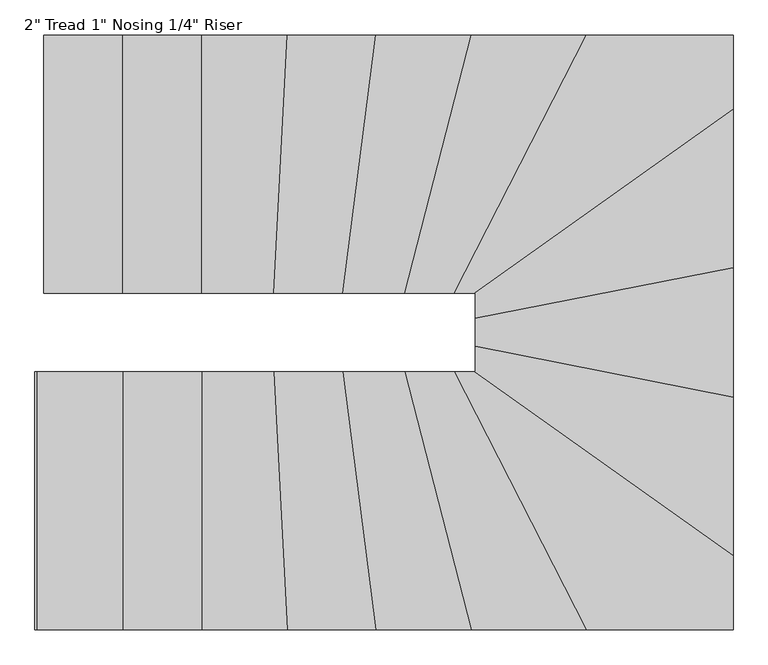
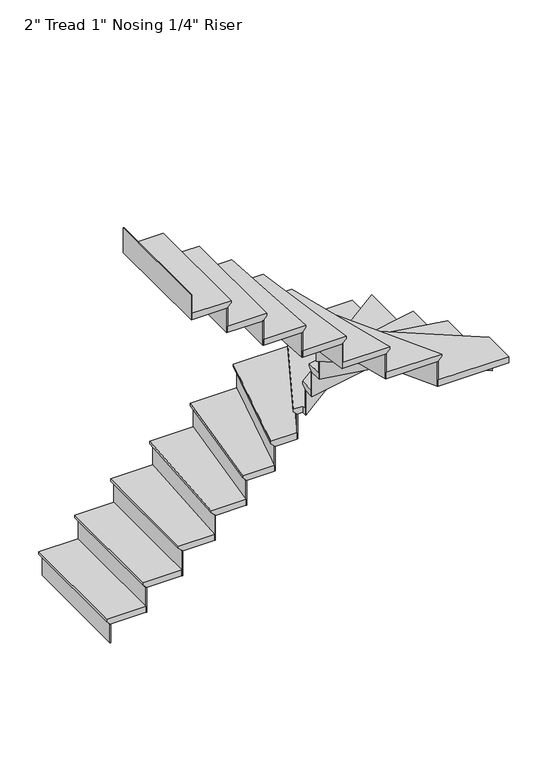
"""IFC4 building model written with IfcOpenShell, lengths in millimetres: stair flight geometry."""

from ifc_helpers import new_model, si_unit, origin, place, context, project, spatial, faceted_brep, source, transform, mapped, element, save


def stair_flight_27d53fa0(model_context):
    return source(origin(), model_context, "Body", "Brep", [
        faceted_brep([(306.9570026, -4376.7064015, 6584.95), (306.9570026, -4376.7064015, 6604.0), (306.9570026, -3462.3064015, 6604.0), (306.9570026, -3462.3064015, 6584.95), (332.3570026, -4376.7064015, 6559.55), (332.3570026, -3462.3064015, 6559.55), (611.7570026, -4376.7064015, 6604.0), (611.7570026, -3462.3064015, 6604.0), (332.3570026, -3462.3064015, 6553.2), (611.7570026, -3462.3064015, 6553.2), (611.7570026, -4376.7064015, 6553.2), (332.3570026, -4376.7064015, 6553.2)], [[[0, 1, 2, 3]], [[4, 0, 3, 5]], [[2, 1, 6, 7]], [[8, 9, 10, 11]], [[2, 7, 9, 8, 5, 3]], [[8, 11, 4, 5]], [[6, 1, 0, 4, 11, 10]], [[7, 6, 10, 9]]]),
        faceted_brep([(332.3570026, -4376.7064015, 6553.2), (332.3570026, -4376.7064015, 6400.8), (338.7070026, -4376.7064015, 6400.8), (338.7070026, -4376.7064015, 6553.2), (332.3570026, -3462.3064015, 6553.2), (338.7070026, -3462.3064015, 6553.2), (338.7070026, -3462.3064015, 6400.8), (332.3570026, -3462.3064015, 6400.8)], [[[0, 1, 2, 3]], [[4, 5, 6, 7]], [[1, 0, 4, 7]], [[2, 1, 7, 6]], [[3, 2, 6, 5]], [[0, 3, 5, 4]]]),
        faceted_brep([(611.7570026, -4376.7064015, 6756.4), (611.7570026, -4376.7064015, 6553.2), (618.1070026, -4376.7064015, 6553.2), (618.1070026, -4376.7064015, 6756.4), (611.7570026, -3462.3064015, 6756.4), (618.1070026, -3462.3064015, 6756.4), (618.1070026, -3462.3064015, 6553.2), (611.7570026, -3462.3064015, 6553.2)], [[[0, 1, 2, 3]], [[4, 5, 6, 7]], [[1, 0, 4, 7]], [[2, 1, 7, 6]], [[3, 2, 6, 5]], [[0, 3, 5, 4]]]),
        faceted_brep([(586.3570026, -3462.3064015, 6807.2), (586.3570026, -4376.7064015, 6807.2), (891.1570026, -4376.7064015, 6807.2), (891.1570026, -3462.3064015, 6807.2), (611.7570026, -3462.3064015, 6756.4), (891.1570026, -3462.3064015, 6756.4), (891.1570026, -4376.7064015, 6756.4), (611.7570026, -4376.7064015, 6756.4), (611.7570026, -3462.3064015, 6762.75), (586.3570026, -3462.3064015, 6788.15), (611.7570026, -4376.7064015, 6762.75), (586.3570026, -4376.7064015, 6788.15)], [[[0, 1, 2, 3]], [[4, 5, 6, 7]], [[0, 3, 5, 4, 8, 9]], [[4, 7, 10, 8]], [[2, 1, 11, 10, 7, 6]], [[3, 2, 6, 5]], [[11, 1, 0, 9]], [[10, 11, 9, 8]]]),
        faceted_brep([(891.1570026, -4376.7064015, 6959.6), (891.1570026, -4376.7064015, 6756.4), (897.5070026, -4376.7064015, 6756.4), (897.5070026, -4376.7064015, 6959.6), (891.1570026, -3462.3064015, 6959.6), (897.5070026, -3462.3064015, 6959.6), (897.5070026, -3462.3064015, 6756.4), (891.1570026, -3462.3064015, 6756.4)], [[[0, 1, 2, 3]], [[4, 5, 6, 7]], [[1, 0, 4, 7]], [[2, 1, 7, 6]], [[3, 2, 6, 5]], [[0, 3, 5, 4]]]),
        faceted_brep([(865.7570026, -3462.3064015, 7010.4), (865.7570026, -4376.7064015, 7010.4), (1146.824164, -4376.7064015, 7010.4), (1194.3584344, -3462.3064015, 7010.4), (891.1570026, -3462.3064015, 6959.6), (1194.3584344, -3462.3064015, 6959.6), (1146.824164, -4376.7064015, 6959.6), (891.1570026, -4376.7064015, 6959.6), (891.1570026, -3462.3064015, 6965.95), (865.7570026, -3462.3064015, 6991.35), (891.1570026, -4376.7064015, 6965.95), (865.7570026, -4376.7064015, 6991.35)], [[[0, 1, 2, 3]], [[4, 5, 6, 7]], [[0, 3, 5, 4, 8, 9]], [[4, 7, 10, 8]], [[2, 1, 11, 10, 7, 6]], [[3, 2, 6, 5]], [[11, 1, 0, 9]], [[10, 11, 9, 8]]]),
        faceted_brep([(1146.824164, -4376.7064015, 7162.8), (1146.824164, -4376.7064015, 6959.6), (1153.1827382, -4376.7064015, 6959.6), (1153.1827382, -4376.7064015, 7162.8), (1194.3584344, -3462.3064015, 7162.8), (1200.7170086, -3462.3064015, 7162.8), (1200.7170086, -3462.3064015, 6959.6), (1194.3584344, -3462.3064015, 6959.6)], [[[0, 1, 2, 3]], [[4, 5, 6, 7]], [[1, 0, 4, 7]], [[2, 1, 7, 6]], [[3, 2, 6, 5]], [[0, 3, 5, 4]]]),
        faceted_brep([(1168.9241378, -3462.3064015, 7213.6), (1121.3898673, -4376.7064015, 7213.6), (1390.9908638, -4376.7064015, 7213.6), (1509.3469155, -3462.3064015, 7213.6), (1194.3584344, -3462.3064015, 7162.8), (1509.3469155, -3462.3064015, 7162.8), (1390.9908638, -4376.7064015, 7162.8), (1146.824164, -4376.7064015, 7162.8), (1194.3584344, -3462.3064015, 7169.15), (1168.9241378, -3462.3064015, 7194.55), (1146.824164, -4376.7064015, 7169.15), (1121.3898673, -4376.7064015, 7194.55)], [[[0, 1, 2, 3]], [[4, 5, 6, 7]], [[0, 3, 5, 4, 8, 9]], [[4, 7, 10, 8]], [[2, 1, 11, 10, 7, 6]], [[3, 2, 6, 5]], [[11, 1, 0, 9]], [[10, 11, 9, 8]]]),
        faceted_brep([(1390.9908638, -4376.7064015, 7366.0), (1390.9908638, -4376.7064015, 7162.8), (1397.3938356, -4376.7064015, 7162.8), (1397.3938356, -4376.7064015, 7366.0), (1509.3469155, -3462.3064015, 7366.0), (1515.7498873, -3462.3064015, 7366.0), (1515.7498873, -3462.3064015, 7162.8), (1509.3469155, -3462.3064015, 7162.8)], [[[0, 1, 2, 3]], [[4, 5, 6, 7]], [[1, 0, 4, 7]], [[2, 1, 7, 6]], [[3, 2, 6, 5]], [[0, 3, 5, 4]]]),
        faceted_brep([(1483.7350284, -3462.3064015, 7416.8), (1365.3789767, -4376.7064015, 7416.8), (1612.6180863, -4376.7064015, 7416.8), (1847.7485337, -3462.3064015, 7416.8), (1509.3469155, -3462.3064015, 7366.0), (1847.7485337, -3462.3064015, 7366.0), (1612.6180863, -4376.7064015, 7366.0), (1390.9908638, -4376.7064015, 7366.0), (1509.3469155, -3462.3064015, 7372.35), (1483.7350284, -3462.3064015, 7397.75), (1390.9908638, -4376.7064015, 7372.35), (1365.3789767, -4376.7064015, 7397.75)], [[[0, 1, 2, 3]], [[4, 5, 6, 7]], [[0, 3, 5, 4, 8, 9]], [[4, 7, 10, 8]], [[2, 1, 11, 10, 7, 6]], [[3, 2, 6, 5]], [[11, 1, 0, 9]], [[10, 11, 9, 8]]]),
        faceted_brep([(1612.6180863, -4376.7064015, 7569.2), (1612.6180863, -4376.7064015, 7366.0), (1619.1746632, -4376.7064015, 7366.0), (1619.1746632, -4376.7064015, 7569.2), (1847.7485337, -3462.3064015, 7569.2), (1854.3051106, -3462.3064015, 7569.2), (1854.3051106, -3462.3064015, 7366.0), (1847.7485337, -3462.3064015, 7366.0)], [[[0, 1, 2, 3]], [[4, 5, 6, 7]], [[1, 0, 4, 7]], [[2, 1, 7, 6]], [[3, 2, 6, 5]], [[0, 3, 5, 4]]]),
        faceted_brep([(1821.5222263, -3462.3064015, 7620.0), (1586.3917788, -4376.7064015, 7620.0), (1788.9647224, -4376.7064015, 7620.0), (2257.7893437, -3462.3064015, 7620.0), (1847.7485337, -3462.3064015, 7569.2), (2257.7893437, -3462.3064015, 7569.2), (1788.9647224, -4376.7064015, 7569.2), (1612.6180863, -4376.7064015, 7569.2), (1847.7485337, -3462.3064015, 7575.55), (1821.5222263, -3462.3064015, 7600.95), (1612.6180863, -4376.7064015, 7575.55), (1586.3917788, -4376.7064015, 7600.95)], [[[0, 1, 2, 3]], [[4, 5, 6, 7]], [[0, 3, 5, 4, 8, 9]], [[4, 7, 10, 8]], [[2, 1, 11, 10, 7, 6]], [[3, 2, 6, 5]], [[11, 1, 0, 9]], [[10, 11, 9, 8]]]),
        faceted_brep([(1788.9647224, -4376.7064015, 7772.4), (1788.9647224, -4376.7064015, 7569.2), (1796.1007055, -4376.7064015, 7569.2), (1796.1007055, -4376.7064015, 7772.4), (2257.7893437, -3462.3064015, 7772.4), (2264.9253269, -3462.3064015, 7772.4), (2264.9253269, -3462.3064015, 7569.2), (2257.7893437, -3462.3064015, 7569.2)], [[[0, 1, 2, 3]], [[4, 5, 6, 7]], [[1, 0, 4, 7]], [[2, 1, 7, 6]], [[3, 2, 6, 5]], [[0, 3, 5, 4]]]),
        faceted_brep([(2749.0886944, -3755.9875352, 7823.2), (2749.0886944, -3462.3064015, 7823.2), (2229.2454112, -3462.3064015, 7823.2), (1760.4207899, -4376.7064015, 7823.2), (1834.6886944, -4376.7064015, 7823.2), (1834.6886944, -4406.2614844, 7823.2), (2749.0886944, -3462.3064015, 7772.4), (2749.0886944, -3755.9875352, 7772.4), (1834.6886944, -4406.2614844, 7772.4), (1834.6886944, -4376.7064015, 7772.4), (1788.9647224, -4376.7064015, 7772.4), (2257.7893437, -3462.3064015, 7772.4), (2257.7893437, -3462.3064015, 7778.75), (2229.2454112, -3462.3064015, 7804.15), (1788.9647224, -4376.7064015, 7778.75), (1760.4207899, -4376.7064015, 7804.15)], [[[0, 1, 2, 3, 4, 5]], [[6, 7, 8, 9, 10, 11]], [[1, 0, 7, 6]], [[2, 1, 6, 11, 12, 13]], [[11, 10, 14, 12]], [[4, 3, 15, 14, 10, 9]], [[5, 4, 9, 8]], [[0, 5, 8, 7]], [[15, 3, 2, 13]], [[14, 15, 13, 12]]]),
        faceted_brep([(1834.6886944, -4406.2614844, 7975.6), (1834.6886944, -4406.2614844, 7772.4), (1834.6886944, -4414.0534592, 7772.4), (1834.6886944, -4414.0534592, 7975.6), (2749.0886944, -3755.9875352, 7975.6), (2749.0886944, -3763.77951, 7975.6), (2749.0886944, -3763.77951, 7772.4), (2749.0886944, -3755.9875352, 7772.4)], [[[0, 1, 2, 3]], [[4, 5, 6, 7]], [[1, 0, 4, 7]], [[2, 1, 7, 6]], [[3, 2, 6, 5]], [[0, 3, 5, 4]]]),
        faceted_brep([(2749.0886944, -3724.819636, 8026.4), (1834.6886944, -4375.0935852, 8026.4), (1834.6886944, -4492.7155714, 8026.4), (2749.0886944, -4312.4747151, 8026.4), (2749.0886944, -3755.9875352, 7975.6), (2749.0886944, -4312.4747151, 7975.6), (1834.6886944, -4492.7155714, 7975.6), (1834.6886944, -4406.2614844, 7975.6), (2749.0886944, -3755.9875352, 7981.95), (2749.0886944, -3724.819636, 8007.35), (1834.6886944, -4406.2614844, 7981.95), (1834.6886944, -4375.0935852, 8007.35)], [[[0, 1, 2, 3]], [[4, 5, 6, 7]], [[0, 3, 5, 4, 8, 9]], [[4, 7, 10, 8]], [[2, 1, 11, 10, 7, 6]], [[3, 2, 6, 5]], [[11, 1, 0, 9]], [[10, 11, 9, 8]]]),
        faceted_brep([(1834.6886944, -4492.7155714, 8178.8), (1834.6886944, -4492.7155714, 7975.6), (1834.6886944, -4499.1877569, 7975.6), (1834.6886944, -4499.1877569, 8178.8), (2749.0886944, -4312.4747151, 8178.8), (2749.0886944, -4318.9469005, 8178.8), (2749.0886944, -4318.9469005, 7975.6), (2749.0886944, -4312.4747151, 7975.6)], [[[0, 1, 2, 3]], [[4, 5, 6, 7]], [[1, 0, 4, 7]], [[2, 1, 7, 6]], [[3, 2, 6, 5]], [[0, 3, 5, 4]]]),
        faceted_brep([(2749.0886944, -4286.5859733, 8229.6), (1834.6886944, -4466.8268297, 8229.6), (1834.6886944, -4591.8747151, 8229.6), (2749.0886944, -4772.1155714, 8229.6), (2749.0886944, -4312.4747151, 8178.8), (2749.0886944, -4772.1155714, 8178.8), (1834.6886944, -4591.8747151, 8178.8), (1834.6886944, -4492.7155714, 8178.8), (2749.0886944, -4312.4747151, 8185.15), (2749.0886944, -4286.5859733, 8210.55), (1834.6886944, -4492.7155714, 8185.15), (1834.6886944, -4466.8268297, 8210.55)], [[[0, 1, 2, 3]], [[4, 5, 6, 7]], [[0, 3, 5, 4, 8, 9]], [[4, 7, 10, 8]], [[2, 1, 11, 10, 7, 6]], [[3, 2, 6, 5]], [[11, 1, 0, 9]], [[10, 11, 9, 8]]]),
        faceted_brep([(1834.6886944, -4591.8747151, 8382.0), (1834.6886944, -4591.8747151, 8178.8), (1834.6886944, -4598.3469005, 8178.8), (1834.6886944, -4598.3469005, 8382.0), (2749.0886944, -4772.1155714, 8382.0), (2749.0886944, -4778.5877569, 8382.0), (2749.0886944, -4778.5877569, 8178.8), (2749.0886944, -4772.1155714, 8178.8)], [[[0, 1, 2, 3]], [[4, 5, 6, 7]], [[1, 0, 4, 7]], [[2, 1, 7, 6]], [[3, 2, 6, 5]], [[0, 3, 5, 4]]]),
        faceted_brep([(2749.0886944, -4746.2268297, 8432.8), (1834.6886944, -4565.9859733, 8432.8), (1834.6886944, -4656.1064015, 8432.8), (1788.5932199, -4656.1064015, 8432.8), (2749.0886944, -5339.1610662, 8432.8), (2749.0886944, -4772.1155714, 8382.0), (2749.0886944, -5339.1610662, 8382.0), (1788.5932199, -4656.1064015, 8382.0), (1834.6886944, -4656.1064015, 8382.0), (1834.6886944, -4591.8747151, 8382.0), (2749.0886944, -4772.1155714, 8388.35), (2749.0886944, -4746.2268297, 8413.75), (1834.6886944, -4591.8747151, 8388.35), (1834.6886944, -4565.9859733, 8413.75)], [[[0, 1, 2, 3, 4]], [[5, 6, 7, 8, 9]], [[0, 4, 6, 5, 10, 11]], [[5, 9, 12, 10]], [[2, 1, 13, 12, 9, 8]], [[3, 2, 8, 7]], [[4, 3, 7, 6]], [[13, 1, 0, 11]], [[12, 13, 11, 10]]]),
        faceted_brep([(1788.5932199, -4656.1064015, 8585.2), (1788.5932199, -4656.1064015, 8382.0), (1777.6363274, -4656.1064015, 8382.0), (1777.6363274, -4656.1064015, 8585.2), (2749.0886944, -5339.1610662, 8585.2), (2749.0886944, -5346.953041, 8585.2), (2749.0886944, -5346.953041, 8382.0), (2749.0886944, -5339.1610662, 8382.0)], [[[0, 1, 2, 3]], [[4, 5, 6, 7]], [[1, 0, 4, 7]], [[2, 1, 7, 6]], [[3, 2, 6, 5]], [[0, 3, 5, 4]]]),
        faceted_brep([(2200.7014787, -5570.5064015, 8636.0), (2749.0886944, -5570.5064015, 8636.0), (2749.0886944, -5307.993167, 8636.0), (1832.4207899, -4656.1064015, 8636.0), (1731.8768573, -4656.1064015, 8636.0), (2749.0886944, -5570.5064015, 8585.2), (2200.7014787, -5570.5064015, 8585.2), (1731.8768573, -4656.1064015, 8585.2), (1788.5932199, -4656.1064015, 8585.2), (2749.0886944, -5339.1610662, 8585.2), (2749.0886944, -5339.1610662, 8591.55), (2749.0886944, -5307.993167, 8616.95), (1788.5932199, -4656.1064015, 8591.55), (1832.4207899, -4656.1064015, 8616.95)], [[[0, 1, 2, 3, 4]], [[5, 6, 7, 8, 9]], [[1, 0, 6, 5]], [[2, 1, 5, 9, 10, 11]], [[9, 8, 12, 10]], [[4, 3, 13, 12, 8, 7]], [[0, 4, 7, 6]], [[13, 3, 2, 11]], [[12, 13, 11, 10]]]),
        faceted_brep([(1731.8768573, -4656.1064015, 8788.4), (1731.8768573, -4656.1064015, 8585.2), (1724.7408742, -4656.1064015, 8585.2), (1724.7408742, -4656.1064015, 8788.4), (2200.7014787, -5570.5064015, 8788.4), (2193.5654955, -5570.5064015, 8788.4), (2193.5654955, -5570.5064015, 8585.2), (2200.7014787, -5570.5064015, 8585.2)], [[[0, 1, 2, 3]], [[4, 5, 6, 7]], [[1, 0, 4, 7]], [[2, 1, 7, 6]], [[3, 2, 6, 5]], [[0, 3, 5, 4]]]),
        faceted_brep([(2229.2454112, -5570.5064015, 8839.2), (1760.4207899, -4656.1064015, 8839.2), (1560.1654714, -4656.1064015, 8839.2), (1795.2959188, -5570.5064015, 8839.2), (2200.7014787, -5570.5064015, 8788.4), (1795.2959188, -5570.5064015, 8788.4), (1560.1654714, -4656.1064015, 8788.4), (1731.8768573, -4656.1064015, 8788.4), (2200.7014787, -5570.5064015, 8794.75), (2229.2454112, -5570.5064015, 8820.15), (1731.8768573, -4656.1064015, 8794.75), (1760.4207899, -4656.1064015, 8820.15)], [[[0, 1, 2, 3]], [[4, 5, 6, 7]], [[0, 3, 5, 4, 8, 9]], [[4, 7, 10, 8]], [[2, 1, 11, 10, 7, 6]], [[3, 2, 6, 5]], [[11, 1, 0, 9]], [[10, 11, 9, 8]]]),
        faceted_brep([(1560.1654714, -4656.1064015, 8991.6), (1560.1654714, -4656.1064015, 8788.4), (1553.6088945, -4656.1064015, 8788.4), (1553.6088945, -4656.1064015, 8991.6), (1795.2959188, -5570.5064015, 8991.6), (1788.7393419, -5570.5064015, 8991.6), (1788.7393419, -5570.5064015, 8788.4), (1795.2959188, -5570.5064015, 8788.4)], [[[0, 1, 2, 3]], [[4, 5, 6, 7]], [[1, 0, 4, 7]], [[2, 1, 7, 6]], [[3, 2, 6, 5]], [[0, 3, 5, 4]]]),
        faceted_brep([(1821.5222263, -5570.5064015, 9042.4), (1586.3917788, -4656.1064015, 9042.4), (1339.7670896, -4656.1064015, 9042.4), (1458.1231413, -5570.5064015, 9042.4), (1795.2959188, -5570.5064015, 8991.6), (1458.1231413, -5570.5064015, 8991.6), (1339.7670896, -4656.1064015, 8991.6), (1560.1654714, -4656.1064015, 8991.6), (1795.2959188, -5570.5064015, 8997.95), (1821.5222263, -5570.5064015, 9023.35), (1560.1654714, -4656.1064015, 8997.95), (1586.3917788, -4656.1064015, 9023.35)], [[[0, 1, 2, 3]], [[4, 5, 6, 7]], [[0, 3, 5, 4, 8, 9]], [[4, 7, 10, 8]], [[2, 1, 11, 10, 7, 6]], [[3, 2, 6, 5]], [[11, 1, 0, 9]], [[10, 11, 9, 8]]]),
        faceted_brep([(1339.7670896, -4656.1064015, 9194.8), (1339.7670896, -4656.1064015, 8991.6), (1333.3641178, -4656.1064015, 8991.6), (1333.3641178, -4656.1064015, 9194.8), (1458.1231413, -5570.5064015, 9194.8), (1451.7201695, -5570.5064015, 9194.8), (1451.7201695, -5570.5064015, 8991.6), (1458.1231413, -5570.5064015, 8991.6)], [[[0, 1, 2, 3]], [[4, 5, 6, 7]], [[1, 0, 4, 7]], [[2, 1, 7, 6]], [[3, 2, 6, 5]], [[0, 3, 5, 4]]]),
        faceted_brep([(1483.7350284, -5570.5064015, 9245.6), (1365.3789767, -4656.1064015, 9245.6), (1095.9555707, -4656.1064015, 9245.6), (1143.4898411, -5570.5064015, 9245.6), (1458.1231413, -5570.5064015, 9194.8), (1143.4898411, -5570.5064015, 9194.8), (1095.9555707, -4656.1064015, 9194.8), (1339.7670896, -4656.1064015, 9194.8), (1458.1231413, -5570.5064015, 9201.15), (1483.7350284, -5570.5064015, 9226.55), (1339.7670896, -4656.1064015, 9201.15), (1365.3789767, -4656.1064015, 9226.55)], [[[0, 1, 2, 3]], [[4, 5, 6, 7]], [[0, 3, 5, 4, 8, 9]], [[4, 7, 10, 8]], [[2, 1, 11, 10, 7, 6]], [[3, 2, 6, 5]], [[11, 1, 0, 9]], [[10, 11, 9, 8]]]),
        faceted_brep([(1095.9555707, -4656.1064015, 9398.0), (1095.9555707, -4656.1064015, 9194.8), (1089.5969965, -4656.1064015, 9194.8), (1089.5969965, -4656.1064015, 9398.0), (1143.4898411, -5570.5064015, 9398.0), (1137.1312669, -5570.5064015, 9398.0), (1137.1312669, -5570.5064015, 9194.8), (1143.4898411, -5570.5064015, 9194.8)], [[[0, 1, 2, 3]], [[4, 5, 6, 7]], [[1, 0, 4, 7]], [[2, 1, 7, 6]], [[3, 2, 6, 5]], [[0, 3, 5, 4]]]),
        faceted_brep([(1168.9241378, -5570.5064015, 9448.8), (1121.3898673, -4656.1064015, 9448.8), (840.3570026, -4656.1064015, 9448.8), (840.3570026, -5570.5064015, 9448.8), (1143.4898411, -5570.5064015, 9398.0), (840.3570026, -5570.5064015, 9398.0), (840.3570026, -4656.1064015, 9398.0), (1095.9555707, -4656.1064015, 9398.0), (1143.4898411, -5570.5064015, 9404.35), (1168.9241378, -5570.5064015, 9429.75), (1095.9555707, -4656.1064015, 9404.35), (1121.3898673, -4656.1064015, 9429.75)], [[[0, 1, 2, 3]], [[4, 5, 6, 7]], [[0, 3, 5, 4, 8, 9]], [[4, 7, 10, 8]], [[2, 1, 11, 10, 7, 6]], [[3, 2, 6, 5]], [[11, 1, 0, 9]], [[10, 11, 9, 8]]]),
        faceted_brep([(840.3570026, -4656.1064015, 9601.2), (840.3570026, -4656.1064015, 9398.0), (834.0070026, -4656.1064015, 9398.0), (834.0070026, -4656.1064015, 9601.2), (840.3570026, -5570.5064015, 9601.2), (834.0070026, -5570.5064015, 9601.2), (834.0070026, -5570.5064015, 9398.0), (840.3570026, -5570.5064015, 9398.0)], [[[0, 1, 2, 3]], [[4, 5, 6, 7]], [[1, 0, 4, 7]], [[2, 1, 7, 6]], [[3, 2, 6, 5]], [[0, 3, 5, 4]]]),
        faceted_brep([(865.7570026, -5570.5064015, 9652.0), (865.7570026, -4656.1064015, 9652.0), (560.9570026, -4656.1064015, 9652.0), (560.9570026, -5570.5064015, 9652.0), (840.3570026, -5570.5064015, 9601.2), (560.9570026, -5570.5064015, 9601.2), (560.9570026, -4656.1064015, 9601.2), (840.3570026, -4656.1064015, 9601.2), (840.3570026, -5570.5064015, 9607.55), (865.7570026, -5570.5064015, 9632.95), (840.3570026, -4656.1064015, 9607.55), (865.7570026, -4656.1064015, 9632.95)], [[[0, 1, 2, 3]], [[4, 5, 6, 7]], [[0, 3, 5, 4, 8, 9]], [[4, 7, 10, 8]], [[2, 1, 11, 10, 7, 6]], [[3, 2, 6, 5]], [[11, 1, 0, 9]], [[10, 11, 9, 8]]]),
        faceted_brep([(560.9570026, -4656.1064015, 9804.4), (560.9570026, -4656.1064015, 9601.2), (554.6070026, -4656.1064015, 9601.2), (554.6070026, -4656.1064015, 9804.4), (560.9570026, -5570.5064015, 9804.4), (554.6070026, -5570.5064015, 9804.4), (554.6070026, -5570.5064015, 9601.2), (560.9570026, -5570.5064015, 9601.2)], [[[0, 1, 2, 3]], [[4, 5, 6, 7]], [[1, 0, 4, 7]], [[2, 1, 7, 6]], [[3, 2, 6, 5]], [[0, 3, 5, 4]]]),
        faceted_brep([(281.5570026, -4656.1064015, 10007.6), (281.5570026, -4656.1064015, 9804.4), (275.2070026, -4656.1064015, 9804.4), (275.2070026, -4656.1064015, 10007.6), (281.5570026, -5570.5064015, 10007.6), (275.2070026, -5570.5064015, 10007.6), (275.2070026, -5570.5064015, 9804.4), (281.5570026, -5570.5064015, 9804.4)], [[[0, 1, 2, 3]], [[4, 5, 6, 7]], [[1, 0, 4, 7]], [[2, 1, 7, 6]], [[3, 2, 6, 5]], [[0, 3, 5, 4]]]),
        faceted_brep([(586.3570026, -5570.5064015, 9855.2), (586.3570026, -4656.1064015, 9855.2), (281.5570026, -4656.1064015, 9855.2), (281.5570026, -5570.5064015, 9855.2), (560.9570026, -5570.5064015, 9804.4), (281.5570026, -5570.5064015, 9804.4), (281.5570026, -4656.1064015, 9804.4), (560.9570026, -4656.1064015, 9804.4), (560.9570026, -5570.5064015, 9810.75), (586.3570026, -5570.5064015, 9836.15), (560.9570026, -4656.1064015, 9810.75), (586.3570026, -4656.1064015, 9836.15)], [[[0, 1, 2, 3]], [[4, 5, 6, 7]], [[0, 3, 5, 4, 8, 9]], [[4, 7, 10, 8]], [[2, 1, 11, 10, 7, 6]], [[3, 2, 6, 5]], [[11, 1, 0, 9]], [[10, 11, 9, 8]]]),
    ])


if __name__ == "__main__":
    model = new_model("IFC4")
    model_context = context("Model", 3, world=origin())
    ifc_project = project(units=[si_unit("LENGTHUNIT", "METRE", prefix="MILLI")], contexts=[model_context])
    site = spatial("IfcSite", under=ifc_project)
    building = spatial("IfcBuilding", under=site)
    placement = place(None, origin())
    stair_flight_shape = stair_flight_27d53fa0(model_context)
    element("IfcStairFlight", 1, ObjectType="2\" Tread 1\" Nosing 1/4\" Riser", at=placement, inside=building, context=model_context, shape_type="MappedRepresentation", body=[
        mapped(stair_flight_shape, transform((0.0, 0.0, 0.0), x_axis=(1.0, 0.0, 0.0), y_axis=(0.0, 1.0, 0.0), z_axis=(0.0, 0.0, 1.0))),
    ])
    save(model, "model.ifc")
